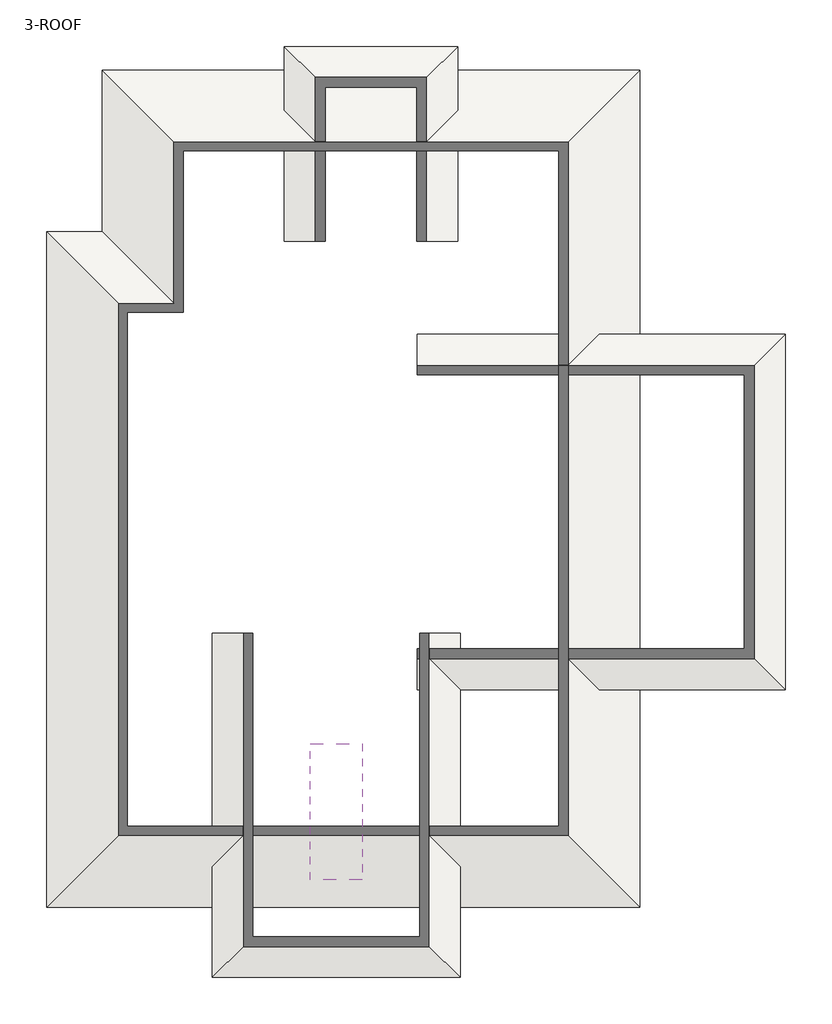
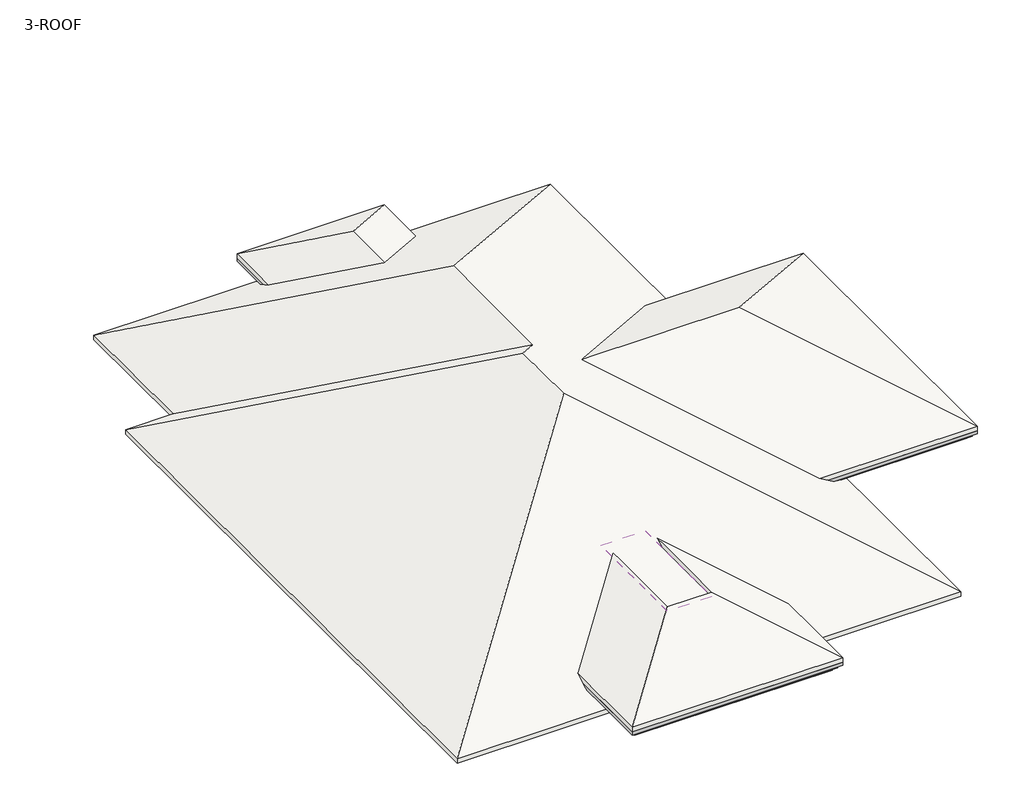
# One storey: 5 roofs, 3 furniture elements.
"""IFC4 building model written with IfcOpenShell, lengths in millimetres."""

from ifc_helpers import new_model, si_unit, frame, origin, place, context, project, spatial, polyline, outline, extrude, faceted_brep, transform, mapped, element, save
from components import casework_4_casework_4_96edb60c, casework_5_casework_5_052b1e20, casework_6_casework_6_bf376347

model = new_model("IFC4")

# Units and contexts
model_context = context("Model", 3, world=origin())
ifc_project = project(units=[si_unit("LENGTHUNIT", "METRE", prefix="MILLI")], contexts=[model_context])

# Site, building, storey
site = spatial("IfcSite", under=ifc_project)
building = spatial("IfcBuilding", under=site)
storey = spatial("IfcBuildingStorey", under=building, Name="3-ROOF", Elevation=4050.0)

# Furniture
placement = place(None, origin())
casework_4_casework_4_shape = casework_4_casework_4_96edb60c(model_context)
element("IfcFurniture", 1, ObjectType="Casework 4 : Casework 4", at=placement, inside=storey, context=model_context, shape_type="MappedRepresentation", body=[
    mapped(casework_4_casework_4_shape, transform((0.0, 0.0, 0.0), x_axis=(1.0, 0.0, 0.0), y_axis=(0.0, 1.0, 0.0), z_axis=(0.0, 0.0, 1.0))),
])
casework_5_casework_5_shape = casework_5_casework_5_052b1e20(model_context)
element("IfcFurniture", 2, ObjectType="Casework 5 : Casework 5", at=placement, inside=storey, context=model_context, shape_type="MappedRepresentation", body=[
    mapped(casework_5_casework_5_shape, transform((0.0, 0.0, 0.0), x_axis=(1.0, 0.0, 0.0), y_axis=(0.0, 1.0, 0.0), z_axis=(0.0, 0.0, 1.0))),
])
casework_6_casework_6_shape = casework_6_casework_6_bf376347(model_context)
element("IfcFurniture", 3, ObjectType="Casework 6 : Casework 6", at=placement, inside=storey, context=model_context, shape_type="MappedRepresentation", body=[
    mapped(casework_6_casework_6_shape, transform((0.0, 0.0, 0.0), x_axis=(1.0, 0.0, 0.0), y_axis=(0.0, 1.0, 0.0), z_axis=(0.0, 0.0, 1.0))),
])

# Roofs
element("IfcRoof", 4, ObjectType="roof", at=placement, inside=storey, context=model_context, shape_type="Brep", body=[
    faceted_brep([(863.2046034, -4121.6929163, 8423.4282891), (-6711.7953966, -11696.6929163, 4050.0), (-6711.7953966, 5565.8070837, 4050.0), (863.2046034, -2009.1929163, 8423.4282891), (8438.2046034, 9690.8070837, 4050.0), (1575.7046034, 2828.3070837, 8012.0662223), (-5286.7953966, 9690.8070837, 4050.0), (8438.2046034, -11696.6929163, 4050.0), (1575.7046034, -1296.6929163, 8012.0662223), (-5286.7953966, 5565.8070837, 4050.0), (-6711.7953966, -11696.6929163, 4194.3375673), (863.2046034, -4121.6929163, 8567.7658564), (863.2046034, -2009.1929163, 8567.7658564), (-6711.7953966, 5565.8070837, 4194.3375673), (8438.2046034, 9690.8070837, 4194.3375673), (-5286.7953966, 9690.8070837, 4194.3375673), (1575.7046034, 2828.3070837, 8156.4037896), (8438.2046034, -11696.6929163, 4194.3375673), (1575.7046034, -1296.6929163, 8156.4037896), (-5286.7953966, 5565.8070837, 4194.3375673)], [[[0, 1, 2, 3]], [[4, 5, 6]], [[1, 0, 7]], [[7, 0, 3, 8, 5, 4]], [[6, 5, 8, 9]], [[2, 9, 8, 3]], [[10, 11, 12, 13]], [[14, 15, 16]], [[10, 17, 11]], [[17, 14, 16, 18, 12, 11]], [[15, 19, 18, 16]], [[19, 13, 12, 18]], [[7, 17, 10, 1]], [[4, 14, 17, 7]], [[6, 15, 14, 4]], [[9, 19, 15, 6]], [[2, 13, 19, 9]], [[1, 10, 13, 2]]]),
])
element("IfcRoof", 5, ObjectType="roof", at=placement, inside=storey, context=model_context, shape_type="Brep", body=[
    faceted_brep([(688.2046034, -4696.6929163, 6478.7569777), (3855.7046034, -4696.6929163, 4650.0), (3855.7046034, -13486.6929163, 4650.0), (1355.7046034, -10986.6929163, 6093.375673), (1355.7046034, -5696.6929163, 6093.375673), (688.2046034, -5696.6929163, 6478.7569777), (-2479.2953966, -13486.6929163, 4650.0), (20.7046034, -10986.6929163, 6093.375673), (-2479.2953966, -4696.6929163, 4650.0), (20.7046034, -5696.6929163, 6093.375673), (3855.7046034, -4696.6929163, 4794.3375673), (688.2046034, -4696.6929163, 6623.094545), (688.2046034, -5696.6929163, 6623.094545), (1355.7046034, -5696.6929163, 6237.7132403), (1355.7046034, -10986.6929163, 6237.7132403), (3855.7046034, -13486.6929163, 4794.3375673), (-2479.2953966, -13486.6929163, 4794.3375673), (20.7046034, -10986.6929163, 6237.7132403), (-2479.2953966, -4696.6929163, 4794.3375673), (20.7046034, -5696.6929163, 6237.7132403)], [[[0, 1, 2, 3, 4, 5]], [[2, 6, 7, 3]], [[8, 0, 5, 9, 7, 6]], [[10, 11, 12, 13, 14, 15]], [[16, 15, 14, 17]], [[18, 16, 17, 19, 12, 11]], [[16, 18, 8, 6]], [[15, 16, 6, 2]], [[10, 15, 2, 1]], [[1, 0, 8, 18, 11, 10]], [[17, 7, 9, 19]], [[19, 9, 5, 4, 13, 12]], [[3, 14, 13, 4]], [[14, 3, 7, 17]]]),
])
element("IfcRoof", 6, ObjectType="roof", at=placement, inside=storey, context=model_context, shape_type="Brep", body=[
    faceted_brep([(2750.7046034, -1596.6929163, 7269.7268464), (2750.7046034, 2940.8070837, 4650.0), (12150.7046034, 2940.8070837, 4650.0), (7613.2046034, -1596.6929163, 7269.7268464), (12150.7046034, -6134.1929163, 4650.0), (2750.7046034, -6134.1929163, 4650.0), (2750.7046034, 2940.8070837, 4794.3375673), (2750.7046034, -1596.6929163, 7414.0644137), (7613.2046034, -1596.6929163, 7414.0644137), (12150.7046034, 2940.8070837, 4794.3375673), (12150.7046034, -6134.1929163, 4794.3375673), (2750.7046034, -6134.1929163, 4794.3375673)], [[[0, 1, 2, 3]], [[4, 3, 2]], [[5, 0, 3, 4]], [[6, 7, 8, 9]], [[10, 9, 8]], [[11, 10, 8, 7]], [[4, 10, 11, 5]], [[2, 9, 10, 4]], [[1, 6, 9, 2]], [[11, 7, 6, 1, 0, 5]]]),
])
element("IfcRoof", 7, ObjectType="roof", at=placement, inside=storey, context=model_context, shape_type="Brep", body=[
    faceted_brep([(1575.7046034, 5315.8070837, 5927.3874706), (-636.7953966, 5315.8070837, 4650.0), (-636.7953966, 10290.8070837, 4650.0), (1575.7046034, 8078.3070837, 5927.3874706), (3788.2046034, 10290.8070837, 4650.0), (3788.2046034, 5315.8070837, 4650.0), (-636.7953966, 5315.8070837, 4794.3375673), (1575.7046034, 5315.8070837, 6071.7250379), (1575.7046034, 8078.3070837, 6071.7250379), (-636.7953966, 10290.8070837, 4794.3375673), (3788.2046034, 10290.8070837, 4794.3375673), (3788.2046034, 5315.8070837, 4794.3375673)], [[[0, 1, 2, 3]], [[4, 3, 2]], [[5, 0, 3, 4]], [[6, 7, 8, 9]], [[10, 9, 8]], [[11, 10, 8, 7]], [[4, 10, 11, 5]], [[2, 9, 10, 4]], [[1, 6, 9, 2]], [[11, 7, 6, 1, 0, 5]]]),
])
element("IfcRoof", 8, ObjectType="roof", at=placement, inside=storey, context=model_context, shape_type="SweptSolid", body=[
    extrude(outline(polyline([(6237.7132403, 1355.7046034), (6623.094545, 688.2046034), (6237.7132403, 20.7046034), (6093.375673, 20.7046034), (6478.7569777, 688.2046034), (6093.375673, 1355.7046034), (6237.7132403, 1355.7046034)])), frame((0.0, -10986.6929163, 0.0), z_axis=(0.0, 1.0, 0.0), x_axis=(0.0, 0.0, 1.0)), (0.0, 0.0, 1.0), 3468.5855192),
])

save(model, "model.ifc")

# Revit data of these elements
# Type "roof"
#   Layers, outside or top first: 125 mm "roof" (function 1)
# Element 1 (IfcFurniture, "Casework 4 : Casework 4")
#   Phase Created = New Construction
# Element 2 (IfcFurniture, "Casework 5 : Casework 5")
#   Phase Created = New Construction
# Element 3 (IfcFurniture, "Casework 6 : Casework 6")
#   Phase Created = New Construction
# Element 4 (IfcRoof, "roof")
#   built-in parameter 1001705 = 28.1095 (stored number, unit not read)
#   built-in parameter 1001710 = 33615
#   Phase Created = New Construction
#   Materials on its faces: "roof"
# Element 5 (IfcRoof, "roof")
#   built-in parameter 1001705 = 21.7293 (stored number, unit not read)
#   built-in parameter 1001701 = 1.9685 (stored number, unit not read)
#   built-in parameter 1001710 = 33615
#   Phase Created = New Construction
#   Materials on its faces: "roof"
# Element 6 (IfcRoof, "roof")
#   built-in parameter 1001705 = 24.3244 (stored number, unit not read)
#   built-in parameter 1001701 = 1.9685 (stored number, unit not read)
#   built-in parameter 1001710 = 33615
#   Phase Created = New Construction
#   Materials on its faces: "roof"
# Element 7 (IfcRoof, "roof")
#   built-in parameter 1001705 = 19.9204 (stored number, unit not read)
#   built-in parameter 1001701 = 1.9685 (stored number, unit not read)
#   built-in parameter 1001710 = 33615
#   Phase Created = New Construction
#   Materials on its faces: "roof"
# Element 8 (IfcRoof, "roof")
#   built-in parameter 1001705 = 21.7293 (stored number, unit not read)
#   built-in parameter 1001701 = 6.70399 (stored number, unit not read)
#   built-in parameter 1001710 = 33615
#   Phase Created = New Construction
#   Materials on its faces: "roof"
# Materials
#   "roof": class "Generic", colour RGB 86 51 40, transparency 0, Cost = 0
